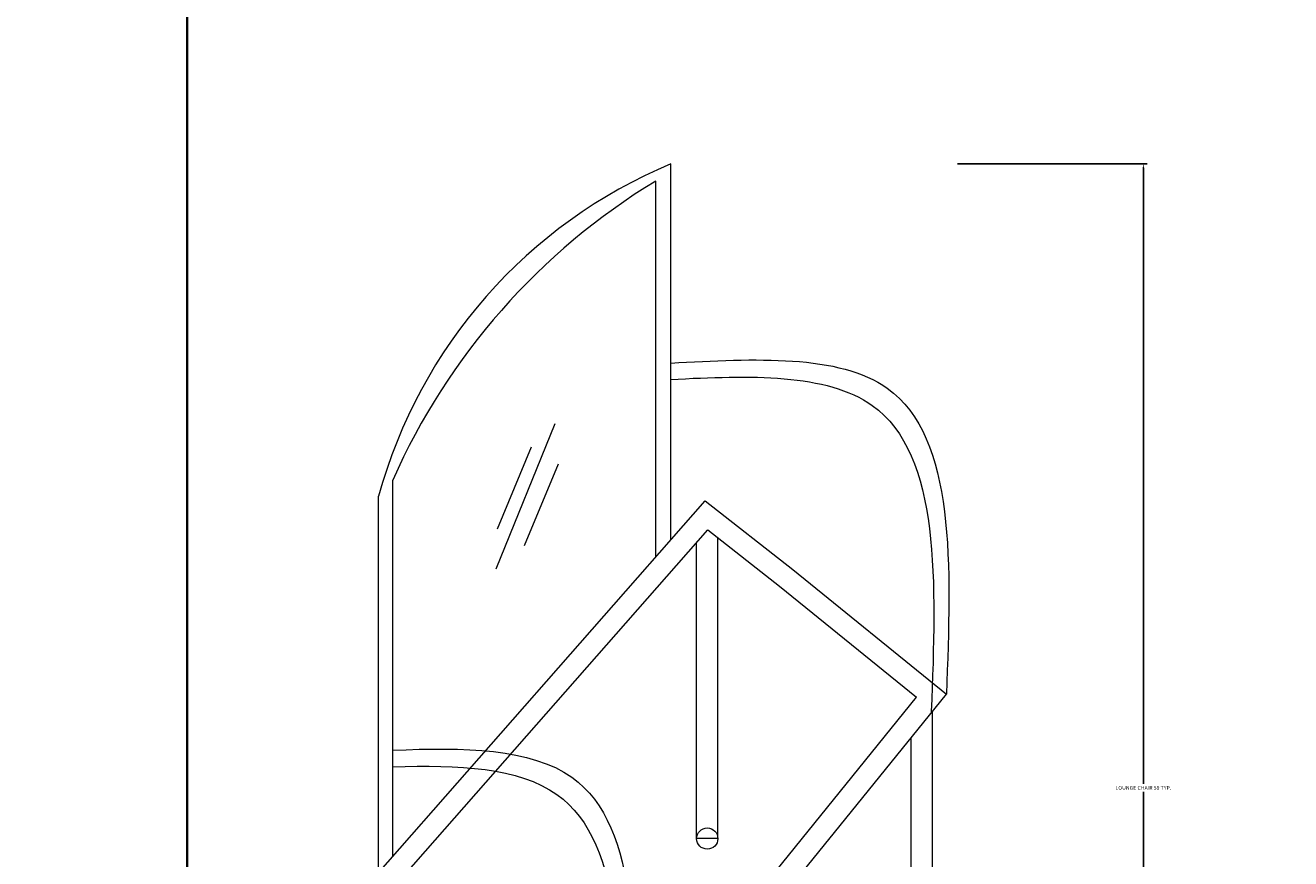
# Model space of a CAD drawing. Units: inches. Extents: x -61 to 1599, y -1316 to 257.
# Tile 17 of 204: x 16 to 76, y -829 to -790. Entities that reach past the tile are written whole.
import ezdxf

# ---------------------------------------------------------------- set-up
doc = ezdxf.new("R2010")
doc.units = ezdxf.units.IN
doc.header["$MEASUREMENT"] = 0
for name, color, linetype, lineweight in [('A-ANNO-DIMS', 2, 'Continuous', 18), ('FURNITURE', 83, 'Continuous', 18), ('WALLS', 4, 'Continuous', 35)]:
    doc.layers.add(name, color=color, linetype=linetype, lineweight=lineweight)
doc.styles.get("Standard").update_dxf_attribs({"font": 'arial.ttf'})
doc.dimstyles.get("Standard").update_dxf_attribs({"dimtxt": 0.18, "dimasz": 0.18, "dimexe": 0.18, "dimexo": 0.0625, "dimgap": 0.09, "dimtad": 0, "dimtih": 1, "dimtoh": 1, "dimdec": 0, "dimzin": 0, "dimdsep": 46, "dimlunit": 3, "dimtxsty": 'Standard', "dimcen": 0.09, "dimadec": 0, "dimazin": 0, "dimtfac": 1, "dimtdec": 0, "dimtofl": 0, "dimtmove": 0, "dimatfit": 3, "dimfxl": 1, "dimtolj": 1, "dimtzin": 0, "dimarcsym": 0})

# ---------------------------------------------------------------- blocks, each defined once
blk = doc.blocks.new('LOUNGE-CHAIR')
for p, q in [((14.756, 41.139), (14.756, 58.888)), ((14.044, 40.329), (14.044, 58.079)), ((6.516, 39.777), (9.293, 46.646)), ((6.577, 41.676), (8.182, 45.543)), ((7.843, 40.874), (9.448, 44.741)), ((1.64, 26.221), (1.64, 43.97)), ((0.966, 25.454), (0.966, 43.203)), ((0.966, 25.454), (0.966, 43.203)), ((0, 24.355), (16.378, 42.984)), ((16.378, 42.984), (20.505, 39.744)), ((16.972, 42.518), (16.972, 42.522)), ((1.449, 24.488), (16.505, 41.614)), ((16.505, 41.614), (19.887, 38.957)), ((16.972, 27.053), (16.972, 41.247)), ((15.972, 27.053), (15.972, 41.008)), ((20.505, 39.744), (27.757, 33.866)), ((19.875, 38.967), (26.35, 33.719)), ((12.015, 16.032), (26.35, 33.719)), ((12.162, 14.625), (27.757, 33.866)), ((27.098, 20.023), (27.098, 33.052)), ((26.098, 20.023), (26.098, 31.819)), ((16.972, 27.053), (15.972, 27.053)), ((1.449, 24.488), (5.717, 21.137)), ((0, 24.355), (5.099, 20.35)), ((0.751, 23.694), (0.787, 23.736)), ((1.726, 7.53), (1.726, 22.999)), ((2.726, 7.53), (2.726, 22.214)), ((5.729, 21.127), (12.015, 16.032)), ((5.099, 20.35), (12.162, 14.625)), ((27.098, 20.023), (26.098, 20.023)), ((12.851, 0.5), (12.851, 15.475)), ((11.851, 0.5), (11.851, 14.878)), ((2.726, 7.53), (1.726, 7.53)), ((12.851, 0.5), (11.851, 0.5))]:
    blk.add_line(p, q)
for centre in [(16.472, 27.053), (26.598, 20.023), (2.226, 7.53), (12.351, 0.5)]:
    blk.add_circle(centre, 0.5)
for centre, radius, start, end in [((23.926, 36.921), 23.804, 112.65862, 164.69962), ((30.248, 31.326), 31.278, 121.20302, 156.15522)]:
    blk.add_arc(centre, radius, start, end)
for points, knots in [([(14.756, 49.49), (18.727, 49.705), (28.376, 50.226), (27.986, 39.927), (27.757, 33.866)], [0, 0, 0, 0, 10.281855, 24.983674, 24.983674, 24.983674, 24.983674]), ([(14.756, 48.719), (18.484, 48.914), (27.655, 49.163), (27.275, 39.117), (27.045, 33.056), (27.044, 33.032), (27.043, 33.009), (27.042, 32.985)], [0.614676, 0.614676, 0.614676, 0.614676, 10.281855, 24.983674, 24.983674, 24.983674, 25.041855, 25.041855, 25.041855, 25.041855]), ([(1.64, 31.221), (4.989, 31.369), (13.472, 31.237), (13.106, 21.568), (12.877, 15.507)], [1.527723, 1.527723, 1.527723, 1.527723, 10.281855, 24.983674, 24.983674, 24.983674, 24.983674]), ([(1.64, 30.439), (4.722, 30.546), (12.751, 30.171), (12.394, 20.758), (12.165, 14.697), (12.164, 14.673), (12.163, 14.649), (12.162, 14.625)], [2.150702, 2.150702, 2.150702, 2.150702, 10.281855, 24.983674, 24.983674, 24.983674, 25.041855, 25.041855, 25.041855, 25.041855])]:
    blk.add_open_spline(points, degree=3, knots=knots)
blk = doc.blocks.new('*D630')
at = {"layer": 'A-ANNO-DIMS', "color": 0, "lineweight": -2, "transparency": 16777216}
for p, q in [((60.054, -796.178), (69.005, -796.178)), ((68.825, -796.358), (68.825, -825.439)), ((68.825, -854.887), (68.825, -825.806)), ((60.054, -855.067), (69.005, -855.067))]:
    blk.add_line(p, q, dxfattribs=at)
at = {"layer": 'A-ANNO-DIMS', "color": 0, "transparency": 16777216}
for points in [[(68.795, -796.358), (68.855, -796.358), (68.825, -796.178)], [(68.795, -854.887), (68.855, -854.887), (68.825, -855.067)]]:
    blk.add_solid(points, dxfattribs=at)
at = {"layer": 'DEFPOINTS', "color": 0, "transparency": 16777216}
for p in [(59.992, -796.178), (68.825, -796.178), (59.992, -855.067)]:
    blk.add_point(p, dxfattribs=at)
at = {"layer": 'A-ANNO-DIMS', "color": 0, "transparency": 16777216, "insert": (68.825, -825.623), "char_height": 0.18, "attachment_point": 5}
blk.add_mtext('\\A1;LOUNGE CHAIR 59 TYP.', dxfattribs=at)
blk = doc.blocks.new('*D687')
at = {"layer": 'A-ANNO-DIMS', "color": 0, "lineweight": -2, "transparency": 16777216}
for p, q in [((289.418, 181.677), (-61.077, 181.677)), ((-60.897, 181.497), (-60.897, -528.952)), ((-60.897, -1239.765), (-60.897, -529.316)), ((319.64, -1239.945), (-61.077, -1239.945))]:
    blk.add_line(p, q, dxfattribs=at)
at = {"layer": 'A-ANNO-DIMS', "color": 0, "transparency": 16777216}
for points in [[(-60.927, 181.497), (-60.867, 181.497), (-60.897, 181.677)], [(-60.927, -1239.765), (-60.867, -1239.765), (-60.897, -1239.945)]]:
    blk.add_solid(points, dxfattribs=at)
at = {"layer": 'DEFPOINTS', "color": 0, "transparency": 16777216}
for p in [(289.481, 181.677), (-60.897, -1239.945), (319.703, -1239.945)]:
    blk.add_point(p, dxfattribs=at)
at = {"layer": 'A-ANNO-DIMS', "color": 0, "transparency": 16777216, "insert": (-60.897, -529.134), "char_height": 0.18, "attachment_point": 5}
blk.add_mtext('\\A1;1421.6', dxfattribs=at)

msp = doc.modelspace()

# ---------------------------------------------------------------- linework, layer by layer
at = {"layer": 'WALLS'}
msp.add_line((23.7028, -943.9446), (23.7028, -787.9446), dxfattribs=at)

# ---------------------------------------------------------------- block references
at = {"layer": 'FURNITURE'}
msp.add_blockref('LOUNGE-CHAIR', (31.776, -855.0667), dxfattribs=at)

# ---------------------------------------------------------------- dimensions: what is measured, and where the dimension line sits
at = {"layer": 'A-ANNO-DIMS'}
dim = msp.add_linear_dim(base=(-60.8972, -1239.9446), p1=(289.4807, 181.6771), p2=(319.7028, -1239.9446), angle=90, dimstyle='Standard', override={"dimdec": 1, "dimlfac": 1, "dimrnd": 0, "dimzin": 0, "dimdsep": 46, "dimlunit": 2}, dxfattribs=at)
dim.commit()
dim.dimension.update_dxf_attribs({"geometry": '*D687', "text_midpoint": (-60.8972, -529.1337)})
dim = msp.add_linear_dim(base=(68.825, -796.1784), p1=(59.9918, -855.0667), p2=(59.9918, -796.1784), angle=90, text='LOUNGE CHAIR <> TYP.', dimstyle='Standard', override={"dimdec": 0, "dimlfac": 1, "dimrnd": 0, "dimzin": 0, "dimdsep": 46, "dimlunit": 2}, dxfattribs=at)
dim.commit()
dim.dimension.update_dxf_attribs({"geometry": '*D630', "text_midpoint": (68.825, -825.6226)})

doc.saveas('drawing.dxf')
